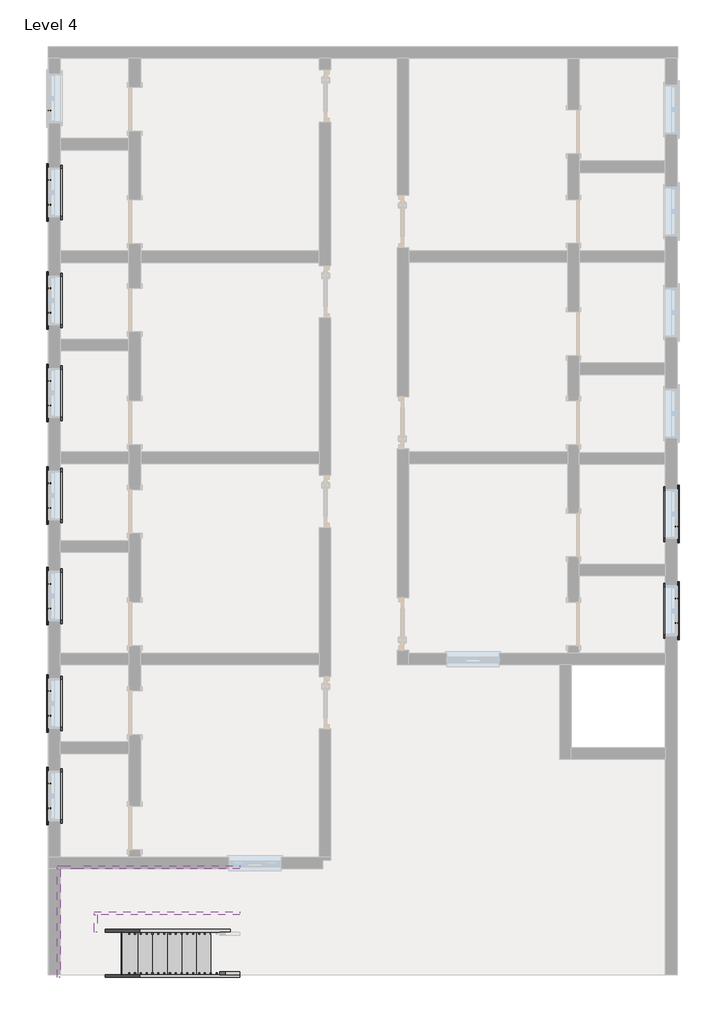
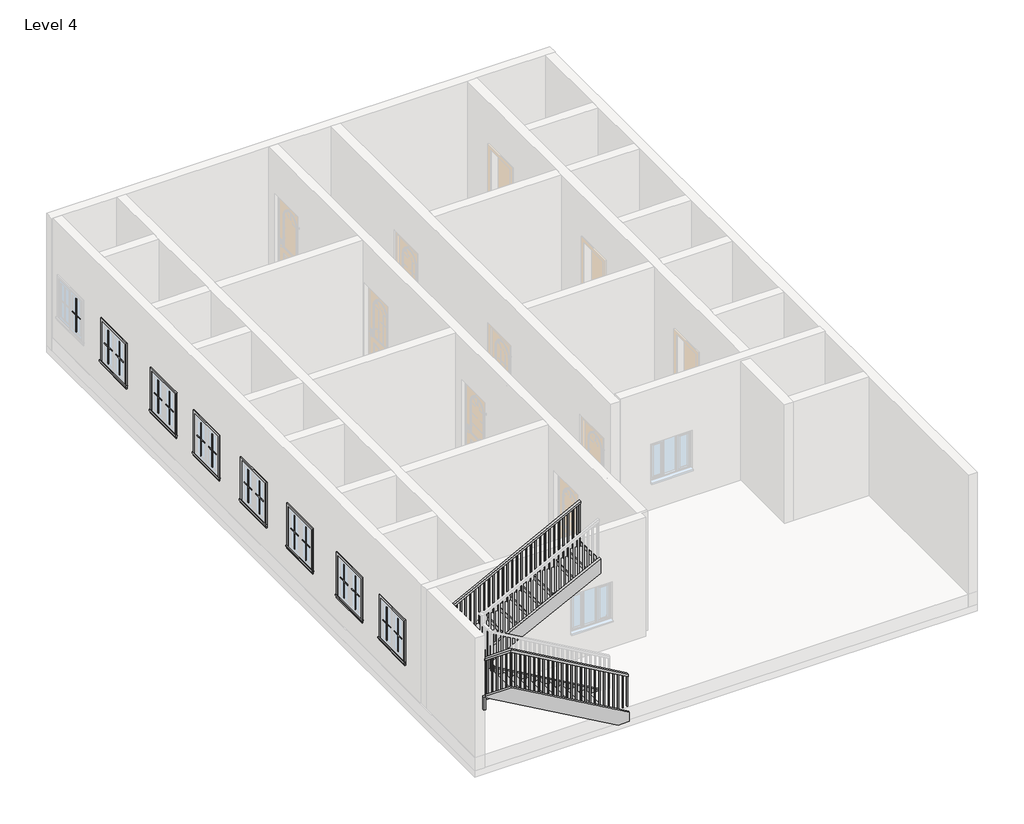
# One storey, part 3 of 4: 36 proxies, 6 members, 1 railing, 1 stair flight.
"""IFC4 building model written with IfcOpenShell, lengths in millimetres."""

from ifc_helpers import new_model, si_unit, frame, origin, place, context, project, spatial, polyline, outline, extrude, faceted_brep, transform, mapped, element, save
from components import muntin_pattern_2x2_muntin_pattern_2x2_b3fe6957, muntin_pattern_2x2_muntin_pattern_2x2_3e0ecaf2, trim_window_exterior_flat_with_sill_41619996, trim_window_interior_flat_picture_frame_51c85655, stair_flight_03342cd4

model = new_model("IFC4")

# Units and contexts
model_context = context("Model", 3, world=origin())
ifc_project = project(units=[si_unit("LENGTHUNIT", "METRE", prefix="MILLI")], contexts=[model_context])

# Site, building, storey
site = spatial("IfcSite", under=ifc_project)
building = spatial("IfcBuilding", under=site)
storey = spatial("IfcBuildingStorey", under=building, Name="Level 4", Elevation=9144.0)

# Proxies
placement = place(None, origin())
muntin_pattern_2x2_muntin_pattern_2x2_shape = muntin_pattern_2x2_muntin_pattern_2x2_b3fe6957(model_context)
element("IfcBuildingElementProxy", 1, Name="Muntin Pattern_2x2 : Muntin Pattern_2x2", ObjectType="Muntin Pattern_2x2 : Muntin Pattern_2x2", at=placement, inside=storey, context=model_context, shape_type="MappedRepresentation", body=[
    mapped(muntin_pattern_2x2_muntin_pattern_2x2_shape, transform((-6438.8858866, 6882.8274728, 10128.25), x_axis=(0.0, 1.0, 0.0), y_axis=(-1.0, 0.0, 0.0), z_axis=(0.0, 0.0, 1.0))),
])
element("IfcBuildingElementProxy", 2, Name="Muntin Pattern_2x2 : Muntin Pattern_2x2", ObjectType="Muntin Pattern_2x2 : Muntin Pattern_2x2", at=placement, inside=storey, context=model_context, shape_type="MappedRepresentation", body=[
    mapped(muntin_pattern_2x2_muntin_pattern_2x2_shape, transform((-6438.8858866, 5244.5274728, 10128.25), x_axis=(0.0, 1.0, 0.0), y_axis=(-1.0, 0.0, 0.0), z_axis=(0.0, 0.0, 1.0))),
])
element("IfcBuildingElementProxy", 3, Name="Muntin Pattern_2x2 : Muntin Pattern_2x2", ObjectType="Muntin Pattern_2x2 : Muntin Pattern_2x2", at=placement, inside=storey, context=model_context, shape_type="MappedRepresentation", body=[
    mapped(muntin_pattern_2x2_muntin_pattern_2x2_shape, transform((-6438.8858866, 3360.4810874, 10128.25), x_axis=(0.0, 1.0, 0.0), y_axis=(-1.0, 0.0, 0.0), z_axis=(0.0, 0.0, 1.0))),
])
element("IfcBuildingElementProxy", 4, Name="Muntin Pattern_2x2 : Muntin Pattern_2x2", ObjectType="Muntin Pattern_2x2 : Muntin Pattern_2x2", at=placement, inside=storey, context=model_context, shape_type="MappedRepresentation", body=[
    mapped(muntin_pattern_2x2_muntin_pattern_2x2_shape, transform((-6438.8858866, 1745.426343, 10128.25), x_axis=(0.0, 1.0, 0.0), y_axis=(-1.0, 0.0, 0.0), z_axis=(0.0, 0.0, 1.0))),
])
element("IfcBuildingElementProxy", 5, Name="Muntin Pattern_2x2 : Muntin Pattern_2x2", ObjectType="Muntin Pattern_2x2 : Muntin Pattern_2x2", at=placement, inside=storey, context=model_context, shape_type="MappedRepresentation", body=[
    mapped(muntin_pattern_2x2_muntin_pattern_2x2_shape, transform((-6438.8858866, -38.6725272, 10128.25), x_axis=(0.0, 1.0, 0.0), y_axis=(-1.0, 0.0, 0.0), z_axis=(0.0, 0.0, 1.0))),
])
element("IfcBuildingElementProxy", 6, Name="Muntin Pattern_2x2 : Muntin Pattern_2x2", ObjectType="Muntin Pattern_2x2 : Muntin Pattern_2x2", at=placement, inside=storey, context=model_context, shape_type="MappedRepresentation", body=[
    mapped(muntin_pattern_2x2_muntin_pattern_2x2_shape, transform((-6438.8858866, -1791.2725272, 10128.25), x_axis=(0.0, 1.0, 0.0), y_axis=(-1.0, 0.0, 0.0), z_axis=(0.0, 0.0, 1.0))),
])
element("IfcBuildingElementProxy", 7, Name="Muntin Pattern_2x2 : Muntin Pattern_2x2", ObjectType="Muntin Pattern_2x2 : Muntin Pattern_2x2", at=placement, inside=storey, context=model_context, shape_type="MappedRepresentation", body=[
    mapped(muntin_pattern_2x2_muntin_pattern_2x2_shape, transform((-6438.8858866, -3658.1725272, 10128.25), x_axis=(0.0, 1.0, 0.0), y_axis=(-1.0, 0.0, 0.0), z_axis=(0.0, 0.0, 1.0))),
])
element("IfcBuildingElementProxy", 8, Name="Muntin Pattern_2x2 : Muntin Pattern_2x2", ObjectType="Muntin Pattern_2x2 : Muntin Pattern_2x2", at=placement, inside=storey, context=model_context, shape_type="MappedRepresentation", body=[
    mapped(muntin_pattern_2x2_muntin_pattern_2x2_shape, transform((-6438.8858866, -5271.0725272, 10128.25), x_axis=(0.0, 1.0, 0.0), y_axis=(-1.0, 0.0, 0.0), z_axis=(0.0, 0.0, 1.0))),
])
element("IfcBuildingElementProxy", 9, Name="Muntin Pattern_2x2 : Muntin Pattern_2x2", ObjectType="Muntin Pattern_2x2 : Muntin Pattern_2x2", at=placement, inside=storey, context=model_context, shape_type="MappedRepresentation", body=[
    mapped(muntin_pattern_2x2_muntin_pattern_2x2_shape, transform((4489.4641134, -1616.6475272, 10128.25), x_axis=(0.0, -1.0, 0.0), y_axis=(1.0, 0.0, 0.0), z_axis=(0.0, 0.0, 1.0))),
])
muntin_pattern_2x2_muntin_pattern_2x2_2_shape = muntin_pattern_2x2_muntin_pattern_2x2_3e0ecaf2(model_context)
element("IfcBuildingElementProxy", 10, Name="Muntin Pattern_2x2 : Muntin Pattern_2x2", ObjectType="Muntin Pattern_2x2 : Muntin Pattern_2x2", at=placement, inside=storey, context=model_context, shape_type="MappedRepresentation", body=[
    mapped(muntin_pattern_2x2_muntin_pattern_2x2_2_shape, transform((-6438.8858866, 5673.1524728, 10128.25), x_axis=(0.0, -1.0, 0.0), y_axis=(1.0, 0.0, 0.0), z_axis=(0.0, 0.0, 1.0))),
])
element("IfcBuildingElementProxy", 11, Name="Muntin Pattern_2x2 : Muntin Pattern_2x2", ObjectType="Muntin Pattern_2x2 : Muntin Pattern_2x2", at=placement, inside=storey, context=model_context, shape_type="MappedRepresentation", body=[
    mapped(muntin_pattern_2x2_muntin_pattern_2x2_2_shape, transform((-6438.8858866, 3789.1060874, 10128.25), x_axis=(0.0, -1.0, 0.0), y_axis=(1.0, 0.0, 0.0), z_axis=(0.0, 0.0, 1.0))),
])
element("IfcBuildingElementProxy", 12, Name="Muntin Pattern_2x2 : Muntin Pattern_2x2", ObjectType="Muntin Pattern_2x2 : Muntin Pattern_2x2", at=placement, inside=storey, context=model_context, shape_type="MappedRepresentation", body=[
    mapped(muntin_pattern_2x2_muntin_pattern_2x2_2_shape, transform((-6438.8858866, 2174.051343, 10128.25), x_axis=(0.0, -1.0, 0.0), y_axis=(1.0, 0.0, 0.0), z_axis=(0.0, 0.0, 1.0))),
])
element("IfcBuildingElementProxy", 13, Name="Muntin Pattern_2x2 : Muntin Pattern_2x2", ObjectType="Muntin Pattern_2x2 : Muntin Pattern_2x2", at=placement, inside=storey, context=model_context, shape_type="MappedRepresentation", body=[
    mapped(muntin_pattern_2x2_muntin_pattern_2x2_2_shape, transform((-6438.8858866, 389.9524728, 10128.25), x_axis=(0.0, -1.0, 0.0), y_axis=(1.0, 0.0, 0.0), z_axis=(0.0, 0.0, 1.0))),
])
element("IfcBuildingElementProxy", 14, Name="Muntin Pattern_2x2 : Muntin Pattern_2x2", ObjectType="Muntin Pattern_2x2 : Muntin Pattern_2x2", at=placement, inside=storey, context=model_context, shape_type="MappedRepresentation", body=[
    mapped(muntin_pattern_2x2_muntin_pattern_2x2_2_shape, transform((-6438.8858866, -1362.6475272, 10128.25), x_axis=(0.0, -1.0, 0.0), y_axis=(1.0, 0.0, 0.0), z_axis=(0.0, 0.0, 1.0))),
])
element("IfcBuildingElementProxy", 15, Name="Muntin Pattern_2x2 : Muntin Pattern_2x2", ObjectType="Muntin Pattern_2x2 : Muntin Pattern_2x2", at=placement, inside=storey, context=model_context, shape_type="MappedRepresentation", body=[
    mapped(muntin_pattern_2x2_muntin_pattern_2x2_2_shape, transform((-6438.8858866, -3229.5475272, 10128.25), x_axis=(0.0, -1.0, 0.0), y_axis=(1.0, 0.0, 0.0), z_axis=(0.0, 0.0, 1.0))),
])
element("IfcBuildingElementProxy", 16, Name="Muntin Pattern_2x2 : Muntin Pattern_2x2", ObjectType="Muntin Pattern_2x2 : Muntin Pattern_2x2", at=placement, inside=storey, context=model_context, shape_type="MappedRepresentation", body=[
    mapped(muntin_pattern_2x2_muntin_pattern_2x2_2_shape, transform((-6438.8858866, -4842.4475272, 10128.25), x_axis=(0.0, -1.0, 0.0), y_axis=(1.0, 0.0, 0.0), z_axis=(0.0, 0.0, 1.0))),
])
element("IfcBuildingElementProxy", 17, Name="Muntin Pattern_2x2 : Muntin Pattern_2x2", ObjectType="Muntin Pattern_2x2 : Muntin Pattern_2x2", at=placement, inside=storey, context=model_context, shape_type="MappedRepresentation", body=[
    mapped(muntin_pattern_2x2_muntin_pattern_2x2_2_shape, transform((4489.4641134, -2045.2725272, 10128.25), x_axis=(0.0, 1.0, 0.0), y_axis=(-1.0, 0.0, 0.0), z_axis=(0.0, 0.0, 1.0))),
])
element("IfcBuildingElementProxy", 18, Name="Muntin Pattern_2x2 : Muntin Pattern_2x2", ObjectType="Muntin Pattern_2x2 : Muntin Pattern_2x2", at=placement, inside=storey, context=model_context, shape_type="MappedRepresentation", body=[
    mapped(muntin_pattern_2x2_muntin_pattern_2x2_2_shape, transform((4489.4641134, -362.5225272, 10128.25), x_axis=(0.0, 1.0, 0.0), y_axis=(-1.0, 0.0, 0.0), z_axis=(0.0, 0.0, 1.0))),
])
trim_window_exterior_flat_with_sill_shape = trim_window_exterior_flat_with_sill_41619996(model_context)
element("IfcBuildingElementProxy", 19, Name="Trim-Window-Exterior-Flat : with Sill", ObjectType="Trim-Window-Exterior-Flat : with Sill", at=placement, inside=storey, context=model_context, shape_type="MappedRepresentation", body=[
    mapped(trim_window_exterior_flat_with_sill_shape, transform((-6448.4108866, 5458.8399728, 10972.8), x_axis=(0.0, -1.0, 0.0), y_axis=(0.0, 0.0, 1.0), z_axis=(-1.0, 0.0, 0.0))),
])
element("IfcBuildingElementProxy", 20, Name="Trim-Window-Exterior-Flat : with Sill", ObjectType="Trim-Window-Exterior-Flat : with Sill", at=placement, inside=storey, context=model_context, shape_type="MappedRepresentation", body=[
    mapped(trim_window_exterior_flat_with_sill_shape, transform((-6448.4108866, 3574.7935874, 10972.8), x_axis=(0.0, -1.0, 0.0), y_axis=(0.0, 0.0, 1.0), z_axis=(-1.0, 0.0, 0.0))),
])
element("IfcBuildingElementProxy", 21, Name="Trim-Window-Exterior-Flat : with Sill", ObjectType="Trim-Window-Exterior-Flat : with Sill", at=placement, inside=storey, context=model_context, shape_type="MappedRepresentation", body=[
    mapped(trim_window_exterior_flat_with_sill_shape, transform((-6448.4108866, 1959.738843, 10972.8), x_axis=(0.0, -1.0, 0.0), y_axis=(0.0, 0.0, 1.0), z_axis=(-1.0, 0.0, 0.0))),
])
element("IfcBuildingElementProxy", 22, Name="Trim-Window-Exterior-Flat : with Sill", ObjectType="Trim-Window-Exterior-Flat : with Sill", at=placement, inside=storey, context=model_context, shape_type="MappedRepresentation", body=[
    mapped(trim_window_exterior_flat_with_sill_shape, transform((-6448.4108866, 175.6399728, 10972.8), x_axis=(0.0, -1.0, 0.0), y_axis=(0.0, 0.0, 1.0), z_axis=(-1.0, 0.0, 0.0))),
])
element("IfcBuildingElementProxy", 23, Name="Trim-Window-Exterior-Flat : with Sill", ObjectType="Trim-Window-Exterior-Flat : with Sill", at=placement, inside=storey, context=model_context, shape_type="MappedRepresentation", body=[
    mapped(trim_window_exterior_flat_with_sill_shape, transform((-6448.4108866, -1576.9600272, 10972.8), x_axis=(0.0, -1.0, 0.0), y_axis=(0.0, 0.0, 1.0), z_axis=(-1.0, 0.0, 0.0))),
])
element("IfcBuildingElementProxy", 24, Name="Trim-Window-Exterior-Flat : with Sill", ObjectType="Trim-Window-Exterior-Flat : with Sill", at=placement, inside=storey, context=model_context, shape_type="MappedRepresentation", body=[
    mapped(trim_window_exterior_flat_with_sill_shape, transform((-6448.4108866, -3443.8600272, 10972.8), x_axis=(0.0, -1.0, 0.0), y_axis=(0.0, 0.0, 1.0), z_axis=(-1.0, 0.0, 0.0))),
])
element("IfcBuildingElementProxy", 25, Name="Trim-Window-Exterior-Flat : with Sill", ObjectType="Trim-Window-Exterior-Flat : with Sill", at=placement, inside=storey, context=model_context, shape_type="MappedRepresentation", body=[
    mapped(trim_window_exterior_flat_with_sill_shape, transform((-6448.4108866, -5056.7600272, 10972.8), x_axis=(0.0, -1.0, 0.0), y_axis=(0.0, 0.0, 1.0), z_axis=(-1.0, 0.0, 0.0))),
])
element("IfcBuildingElementProxy", 26, Name="Trim-Window-Exterior-Flat : with Sill", ObjectType="Trim-Window-Exterior-Flat : with Sill", at=placement, inside=storey, context=model_context, shape_type="MappedRepresentation", body=[
    mapped(trim_window_exterior_flat_with_sill_shape, transform((4498.9891134, -1830.9600272, 10972.8), x_axis=(0.0, 1.0, 0.0), y_axis=(0.0, 0.0, 1.0), z_axis=(1.0, 0.0, 0.0))),
])
element("IfcBuildingElementProxy", 27, Name="Trim-Window-Exterior-Flat : with Sill", ObjectType="Trim-Window-Exterior-Flat : with Sill", at=placement, inside=storey, context=model_context, shape_type="MappedRepresentation", body=[
    mapped(trim_window_exterior_flat_with_sill_shape, transform((4498.9891134, -148.2100272, 10972.8), x_axis=(0.0, 1.0, 0.0), y_axis=(0.0, 0.0, 1.0), z_axis=(1.0, 0.0, 0.0))),
])
trim_window_interior_flat_picture_frame_shape = trim_window_interior_flat_picture_frame_51c85655(model_context)
element("IfcBuildingElementProxy", 28, Name="Trim-Window-Interior-Flat : Picture Frame", ObjectType="Trim-Window-Interior-Flat : Picture Frame", at=placement, inside=storey, context=model_context, shape_type="MappedRepresentation", body=[
    mapped(trim_window_interior_flat_picture_frame_shape, transform((-6245.2108866, 5458.8399728, 10972.8), x_axis=(0.0, 1.0, 0.0), y_axis=(0.0, 0.0, 1.0), z_axis=(1.0, 0.0, 0.0))),
])
element("IfcBuildingElementProxy", 29, Name="Trim-Window-Interior-Flat : Picture Frame", ObjectType="Trim-Window-Interior-Flat : Picture Frame", at=placement, inside=storey, context=model_context, shape_type="MappedRepresentation", body=[
    mapped(trim_window_interior_flat_picture_frame_shape, transform((-6245.2108866, 3574.7935874, 10972.8), x_axis=(0.0, 1.0, 0.0), y_axis=(0.0, 0.0, 1.0), z_axis=(1.0, 0.0, 0.0))),
])
element("IfcBuildingElementProxy", 30, Name="Trim-Window-Interior-Flat : Picture Frame", ObjectType="Trim-Window-Interior-Flat : Picture Frame", at=placement, inside=storey, context=model_context, shape_type="MappedRepresentation", body=[
    mapped(trim_window_interior_flat_picture_frame_shape, transform((-6245.2108866, 1959.738843, 10972.8), x_axis=(0.0, 1.0, 0.0), y_axis=(0.0, 0.0, 1.0), z_axis=(1.0, 0.0, 0.0))),
])
element("IfcBuildingElementProxy", 31, Name="Trim-Window-Interior-Flat : Picture Frame", ObjectType="Trim-Window-Interior-Flat : Picture Frame", at=placement, inside=storey, context=model_context, shape_type="MappedRepresentation", body=[
    mapped(trim_window_interior_flat_picture_frame_shape, transform((-6245.2108866, 175.6399728, 10972.8), x_axis=(0.0, 1.0, 0.0), y_axis=(0.0, 0.0, 1.0), z_axis=(1.0, 0.0, 0.0))),
])
element("IfcBuildingElementProxy", 32, Name="Trim-Window-Interior-Flat : Picture Frame", ObjectType="Trim-Window-Interior-Flat : Picture Frame", at=placement, inside=storey, context=model_context, shape_type="MappedRepresentation", body=[
    mapped(trim_window_interior_flat_picture_frame_shape, transform((-6245.2108866, -1576.9600272, 10972.8), x_axis=(0.0, 1.0, 0.0), y_axis=(0.0, 0.0, 1.0), z_axis=(1.0, 0.0, 0.0))),
])
element("IfcBuildingElementProxy", 33, Name="Trim-Window-Interior-Flat : Picture Frame", ObjectType="Trim-Window-Interior-Flat : Picture Frame", at=placement, inside=storey, context=model_context, shape_type="MappedRepresentation", body=[
    mapped(trim_window_interior_flat_picture_frame_shape, transform((-6245.2108866, -3443.8600272, 10972.8), x_axis=(0.0, 1.0, 0.0), y_axis=(0.0, 0.0, 1.0), z_axis=(1.0, 0.0, 0.0))),
])
element("IfcBuildingElementProxy", 34, Name="Trim-Window-Interior-Flat : Picture Frame", ObjectType="Trim-Window-Interior-Flat : Picture Frame", at=placement, inside=storey, context=model_context, shape_type="MappedRepresentation", body=[
    mapped(trim_window_interior_flat_picture_frame_shape, transform((-6245.2108866, -5056.7600272, 10972.8), x_axis=(0.0, 1.0, 0.0), y_axis=(0.0, 0.0, 1.0), z_axis=(1.0, 0.0, 0.0))),
])
element("IfcBuildingElementProxy", 35, Name="Trim-Window-Interior-Flat : Picture Frame", ObjectType="Trim-Window-Interior-Flat : Picture Frame", at=placement, inside=storey, context=model_context, shape_type="MappedRepresentation", body=[
    mapped(trim_window_interior_flat_picture_frame_shape, transform((4295.7891134, -1830.9600272, 10972.8), x_axis=(0.0, -1.0, 0.0), y_axis=(0.0, 0.0, 1.0), z_axis=(-1.0, 0.0, 0.0))),
])
element("IfcBuildingElementProxy", 36, Name="Trim-Window-Interior-Flat : Picture Frame", ObjectType="Trim-Window-Interior-Flat : Picture Frame", at=placement, inside=storey, context=model_context, shape_type="MappedRepresentation", body=[
    mapped(trim_window_interior_flat_picture_frame_shape, transform((4295.7891134, -148.2100272, 10972.8), x_axis=(0.0, -1.0, 0.0), y_axis=(0.0, 0.0, 1.0), z_axis=(-1.0, 0.0, 0.0))),
])

# Members
element("IfcMember", 37, ObjectType="Stringer - 2\" Width", at=placement, inside=storey, context=model_context, shape_type="SweptSolid", body=[
    extrude(outline(polyline([(9144.0, -3117.2664982), (9352.974685, -3117.2664982), (10816.7714286, -5678.9107995), (10816.7714286, -6245.2108866), (10789.3177409, -6245.2108866), (9144.0, -3365.9048399), (9144.0, -3117.2664982)])), frame((0.0, -8219.0600272, 0.0), z_axis=(0.0, 1.0, 0.0), x_axis=(0.0, 0.0, 1.0)), (0.0, 0.0, 1.0), 50.8),
])
element("IfcMember", 38, ObjectType="Stringer - 2\" Width", at=placement, inside=storey, context=model_context, shape_type="SweptSolid", body=[
    extrude(outline(polyline([(-6245.2108866, -8219.0600272), (-6296.0108866, -8219.0600272), (-6296.0108866, -6326.7600272), (-6245.2108866, -6326.7600272), (-6245.2108866, -8219.0600272)])), frame((0.0, 0.0, 10511.9714286), z_axis=(0.0, 0.0, 1.0), x_axis=(1.0, 0.0, 0.0)), (0.0, 0.0, 1.0), 304.8),
])
element("IfcMember", 39, ObjectType="Stringer - 2\" Width", at=placement, inside=storey, context=model_context, shape_type="SweptSolid", body=[
    extrude(outline(polyline([(10619.8463219, -6296.0108866), (10511.9714286, -6296.0108866), (10511.9714286, -5835.3420022), (11892.5812084, -3117.2664982), (12234.4466461, -3117.2664982), (10619.8463219, -6296.0108866)])), frame((0.0, -6326.7600272, 0.0), z_axis=(0.0, 1.0, 0.0), x_axis=(0.0, 0.0, 1.0)), (0.0, 0.0, 1.0), 50.8),
])
element("IfcMember", 40, ObjectType="Stringer - 2\" Width", at=placement, inside=storey, context=model_context, shape_type="SweptSolid", body=[
    extrude(outline(polyline([(9144.0, -3117.2664982), (9352.974685, -3117.2664982), (10775.374685, -5606.4664982), (10424.3209476, -5606.4664982), (9144.0, -3365.9048399), (9144.0, -3117.2664982)])), frame((0.0, -7431.6600272, 0.0), z_axis=(0.0, 1.0, 0.0), x_axis=(0.0, 0.0, 1.0)), (0.0, 0.0, 1.0), 50.8),
])
element("IfcMember", 41, ObjectType="Stringer - 2\" Width", at=placement, inside=storey, context=model_context, shape_type="SweptSolid", body=[
    extrude(outline(polyline([(-5606.4664982, -7431.6600272), (-5657.2664982, -7431.6600272), (-5657.2664982, -7126.8600272), (-5606.4664982, -7126.8600272), (-5606.4664982, -7431.6600272)])), frame((0.0, 0.0, 10511.9714286), z_axis=(0.0, 0.0, 1.0), x_axis=(1.0, 0.0, 0.0)), (0.0, 0.0, 1.0), 304.8),
])
element("IfcMember", 42, ObjectType="Stringer - 2\" Width", at=placement, inside=storey, context=model_context, shape_type="SweptSolid", body=[
    extrude(outline(polyline([(10944.287916, -5657.2664982), (10602.4224783, -5657.2664982), (11892.5812084, -3117.2664982), (12234.4466461, -3117.2664982), (10944.287916, -5657.2664982)])), frame((0.0, -7126.8600272, 0.0), z_axis=(0.0, 1.0, 0.0), x_axis=(0.0, 0.0, 1.0)), (0.0, 0.0, 1.0), 50.8),
])

# Railing
element("IfcRailing", 43, ObjectType="Handrail - Rectangular", at=placement, inside=storey, context=model_context, shape_type="SolidModel", body=[
    faceted_brep([(-3117.2664982, -8168.2600272, 10203.5428571), (-3117.2664982, -8168.2600272, 10145.0339009), (-3117.2664982, -8117.4600272, 10145.0339009), (-3117.2664982, -8117.4600272, 10203.5428571), (-5657.2664982, -8168.2600272, 11654.9714286), (-5670.7571716, -8168.2600272, 11604.1714286), (-5670.7571716, -8117.4600272, 11604.1714286), (-5657.2664982, -8117.4600272, 11654.9714286), (-6245.2108866, -8168.2600272, 11654.9714286), (-6245.2108866, -8168.2600272, 11604.1714286), (-6194.4108866, -8117.4600272, 11604.1714286), (-6194.4108866, -8117.4600272, 11654.9714286), (-6245.2108866, -6326.7600272, 11654.9714286), (-6245.2108866, -6326.7600272, 11604.1714286), (-6194.4108866, -6377.5600272, 11604.1714286), (-6194.4108866, -6377.5600272, 11654.9714286), (-5939.4887204, -6326.7600272, 11654.9714286), (-5927.1913462, -6326.7600272, 11604.1714286), (-5927.1913462, -6377.5600272, 11604.1714286), (-5939.4887204, -6377.5600272, 11654.9714286), (-3117.2664982, -6326.7600272, 13106.4), (-3117.2664982, -6377.5600272, 13106.4), (-3117.2664982, -6377.5600272, 13049.2756361), (-3117.2664982, -6326.7600272, 13049.2756361)], [[[0, 1, 2, 3]], [[1, 0, 4, 5]], [[2, 1, 5, 6]], [[3, 2, 6, 7]], [[0, 3, 7, 4]], [[5, 4, 8, 9]], [[6, 5, 9, 10]], [[7, 6, 10, 11]], [[4, 7, 11, 8]], [[9, 8, 12, 13]], [[10, 9, 13, 14]], [[11, 10, 14, 15]], [[8, 11, 15, 12]], [[13, 12, 16, 17]], [[14, 13, 17, 18]], [[15, 14, 18, 19]], [[12, 15, 19, 16]], [[20, 21, 22, 23]], [[17, 16, 20, 23]], [[18, 17, 23, 22]], [[19, 18, 22, 21]], [[16, 19, 21, 20]]]),
    extrude(outline(polyline([(13016.325665, -3181.3358866), (12046.8571429, -3181.3358866), (12046.8571429, -3162.2858866), (13026.1228078, -3162.2858866), (13016.325665, -3181.3358866)])), frame((0.0, -6361.6850272, 0.0), z_axis=(0.0, 1.0, 0.0), x_axis=(0.0, 0.0, 1.0)), (0.0, 0.0, 1.0), 19.05),
    extrude(outline(polyline([(12964.0742364, -3282.9358866), (12046.8571429, -3282.9358866), (12046.8571429, -3263.8858866), (12973.8713793, -3263.8858866), (12964.0742364, -3282.9358866)])), frame((0.0, -6361.6850272, 0.0), z_axis=(0.0, 1.0, 0.0), x_axis=(0.0, 0.0, 1.0)), (0.0, 0.0, 1.0), 19.05),
    extrude(outline(polyline([(12911.8228078, -3384.5358866), (11901.7142857, -3384.5358866), (11901.7142857, -3365.4858866), (12921.6199507, -3365.4858866), (12911.8228078, -3384.5358866)])), frame((0.0, -6361.6850272, 0.0), z_axis=(0.0, 1.0, 0.0), x_axis=(0.0, 0.0, 1.0)), (0.0, 0.0, 1.0), 19.05),
    extrude(outline(polyline([(12859.5713793, -3486.1358866), (11901.7142857, -3486.1358866), (11901.7142857, -3467.0858866), (12869.3685221, -3467.0858866), (12859.5713793, -3486.1358866)])), frame((0.0, -6361.6850272, 0.0), z_axis=(0.0, 1.0, 0.0), x_axis=(0.0, 0.0, 1.0)), (0.0, 0.0, 1.0), 19.05),
    extrude(outline(polyline([(12807.3199507, -3587.7358866), (11901.7142857, -3587.7358866), (11901.7142857, -3568.6858866), (12817.1170935, -3568.6858866), (12807.3199507, -3587.7358866)])), frame((0.0, -6361.6850272, 0.0), z_axis=(0.0, 1.0, 0.0), x_axis=(0.0, 0.0, 1.0)), (0.0, 0.0, 1.0), 19.05),
    extrude(outline(polyline([(12755.0685221, -3689.3358866), (11756.5714286, -3689.3358866), (11756.5714286, -3670.2858866), (12764.865665, -3670.2858866), (12755.0685221, -3689.3358866)])), frame((0.0, -6361.6850272, 0.0), z_axis=(0.0, 1.0, 0.0), x_axis=(0.0, 0.0, 1.0)), (0.0, 0.0, 1.0), 19.05),
    extrude(outline(polyline([(12702.8170935, -3790.9358866), (11756.5714286, -3790.9358866), (11756.5714286, -3771.8858866), (12712.6142364, -3771.8858866), (12702.8170935, -3790.9358866)])), frame((0.0, -6361.6850272, 0.0), z_axis=(0.0, 1.0, 0.0), x_axis=(0.0, 0.0, 1.0)), (0.0, 0.0, 1.0), 19.05),
    extrude(outline(polyline([(12650.565665, -3892.5358866), (11756.5714286, -3892.5358866), (11756.5714286, -3873.4858866), (12660.3628078, -3873.4858866), (12650.565665, -3892.5358866)])), frame((0.0, -6361.6850272, 0.0), z_axis=(0.0, 1.0, 0.0), x_axis=(0.0, 0.0, 1.0)), (0.0, 0.0, 1.0), 19.05),
    extrude(outline(polyline([(12598.3142364, -3994.1358866), (11756.5714286, -3994.1358866), (11756.5714286, -3975.0858866), (12608.1113793, -3975.0858866), (12598.3142364, -3994.1358866)])), frame((0.0, -6361.6850272, 0.0), z_axis=(0.0, 1.0, 0.0), x_axis=(0.0, 0.0, 1.0)), (0.0, 0.0, 1.0), 19.05),
    extrude(outline(polyline([(12546.0628078, -4095.7358866), (11756.5714286, -4095.7358866), (11756.5714286, -4076.6858866), (12555.8599507, -4076.6858866), (12546.0628078, -4095.7358866)])), frame((0.0, -6361.6850272, 0.0), z_axis=(0.0, 1.0, 0.0), x_axis=(0.0, 0.0, 1.0)), (0.0, 0.0, 1.0), 19.05),
    extrude(outline(polyline([(12493.8113793, -4197.3358866), (11611.4285714, -4197.3358866), (11611.4285714, -4178.2858866), (12503.6085221, -4178.2858866), (12493.8113793, -4197.3358866)])), frame((0.0, -6361.6850272, 0.0), z_axis=(0.0, 1.0, 0.0), x_axis=(0.0, 0.0, 1.0)), (0.0, 0.0, 1.0), 19.05),
    extrude(outline(polyline([(12441.5599507, -4298.9358866), (11611.4285714, -4298.9358866), (11611.4285714, -4279.8858866), (12451.3570935, -4279.8858866), (12441.5599507, -4298.9358866)])), frame((0.0, -6361.6850272, 0.0), z_axis=(0.0, 1.0, 0.0), x_axis=(0.0, 0.0, 1.0)), (0.0, 0.0, 1.0), 19.05),
    extrude(outline(polyline([(12389.3085221, -4400.5358866), (11466.2857143, -4400.5358866), (11466.2857143, -4381.4858866), (12399.105665, -4381.4858866), (12389.3085221, -4400.5358866)])), frame((0.0, -6361.6850272, 0.0), z_axis=(0.0, 1.0, 0.0), x_axis=(0.0, 0.0, 1.0)), (0.0, 0.0, 1.0), 19.05),
    extrude(outline(polyline([(12337.0570935, -4502.1358866), (11466.2857143, -4502.1358866), (11466.2857143, -4483.0858866), (12346.8542364, -4483.0858866), (12337.0570935, -4502.1358866)])), frame((0.0, -6361.6850272, 0.0), z_axis=(0.0, 1.0, 0.0), x_axis=(0.0, 0.0, 1.0)), (0.0, 0.0, 1.0), 19.05),
    extrude(outline(polyline([(12284.805665, -4603.7358866), (11466.2857143, -4603.7358866), (11466.2857143, -4584.6858866), (12294.6028078, -4584.6858866), (12284.805665, -4603.7358866)])), frame((0.0, -6361.6850272, 0.0), z_axis=(0.0, 1.0, 0.0), x_axis=(0.0, 0.0, 1.0)), (0.0, 0.0, 1.0), 19.05),
    extrude(outline(polyline([(12232.5542364, -4705.3358866), (11321.1428571, -4705.3358866), (11321.1428571, -4686.2858866), (12242.3513793, -4686.2858866), (12232.5542364, -4705.3358866)])), frame((0.0, -6361.6850272, 0.0), z_axis=(0.0, 1.0, 0.0), x_axis=(0.0, 0.0, 1.0)), (0.0, 0.0, 1.0), 19.05),
    extrude(outline(polyline([(12180.3028078, -4806.9358866), (11321.1428571, -4806.9358866), (11321.1428571, -4787.8858866), (12190.0999507, -4787.8858866), (12180.3028078, -4806.9358866)])), frame((0.0, -6361.6850272, 0.0), z_axis=(0.0, 1.0, 0.0), x_axis=(0.0, 0.0, 1.0)), (0.0, 0.0, 1.0), 19.05),
    extrude(outline(polyline([(12128.0513793, -4908.5358866), (11176.0, -4908.5358866), (11176.0, -4889.4858866), (12137.8485221, -4889.4858866), (12128.0513793, -4908.5358866)])), frame((0.0, -6361.6850272, 0.0), z_axis=(0.0, 1.0, 0.0), x_axis=(0.0, 0.0, 1.0)), (0.0, 0.0, 1.0), 19.05),
    extrude(outline(polyline([(12075.7999507, -5010.1358866), (11176.0, -5010.1358866), (11176.0, -4991.0858866), (12085.5970935, -4991.0858866), (12075.7999507, -5010.1358866)])), frame((0.0, -6361.6850272, 0.0), z_axis=(0.0, 1.0, 0.0), x_axis=(0.0, 0.0, 1.0)), (0.0, 0.0, 1.0), 19.05),
    extrude(outline(polyline([(12023.5485221, -5111.7358866), (11176.0, -5111.7358866), (11176.0, -5092.6858866), (12033.345665, -5092.6858866), (12023.5485221, -5111.7358866)])), frame((0.0, -6361.6850272, 0.0), z_axis=(0.0, 1.0, 0.0), x_axis=(0.0, 0.0, 1.0)), (0.0, 0.0, 1.0), 19.05),
    extrude(outline(polyline([(11971.2970935, -5213.3358866), (11030.8571429, -5213.3358866), (11030.8571429, -5194.2858866), (11981.0942364, -5194.2858866), (11971.2970935, -5213.3358866)])), frame((0.0, -6361.6850272, 0.0), z_axis=(0.0, 1.0, 0.0), x_axis=(0.0, 0.0, 1.0)), (0.0, 0.0, 1.0), 19.05),
    extrude(outline(polyline([(11919.045665, -5314.9358866), (11030.8571429, -5314.9358866), (11030.8571429, -5295.8858866), (11928.8428078, -5295.8858866), (11919.045665, -5314.9358866)])), frame((0.0, -6361.6850272, 0.0), z_axis=(0.0, 1.0, 0.0), x_axis=(0.0, 0.0, 1.0)), (0.0, 0.0, 1.0), 19.05),
    extrude(outline(polyline([(11866.7942364, -5416.5358866), (10885.7142857, -5416.5358866), (10885.7142857, -5397.4858866), (11876.5913793, -5397.4858866), (11866.7942364, -5416.5358866)])), frame((0.0, -6361.6850272, 0.0), z_axis=(0.0, 1.0, 0.0), x_axis=(0.0, 0.0, 1.0)), (0.0, 0.0, 1.0), 19.05),
    extrude(outline(polyline([(11814.5428078, -5518.1358866), (10885.7142857, -5518.1358866), (10885.7142857, -5499.0858866), (11824.3399507, -5499.0858866), (11814.5428078, -5518.1358866)])), frame((0.0, -6361.6850272, 0.0), z_axis=(0.0, 1.0, 0.0), x_axis=(0.0, 0.0, 1.0)), (0.0, 0.0, 1.0), 19.05),
    extrude(outline(polyline([(11762.2913793, -5619.7358866), (10885.7142857, -5619.7358866), (10885.7142857, -5600.6858866), (11772.0885221, -5600.6858866), (11762.2913793, -5619.7358866)])), frame((0.0, -6361.6850272, 0.0), z_axis=(0.0, 1.0, 0.0), x_axis=(0.0, 0.0, 1.0)), (0.0, 0.0, 1.0), 19.05),
    extrude(outline(polyline([(11710.0399507, -5721.3358866), (10740.5714286, -5721.3358866), (10740.5714286, -5702.2858866), (11719.8370935, -5702.2858866), (11710.0399507, -5721.3358866)])), frame((0.0, -6361.6850272, 0.0), z_axis=(0.0, 1.0, 0.0), x_axis=(0.0, 0.0, 1.0)), (0.0, 0.0, 1.0), 19.05),
    extrude(outline(polyline([(11657.7885221, -5822.9358866), (10740.5714286, -5822.9358866), (10740.5714286, -5803.8858866), (11667.585665, -5803.8858866), (11657.7885221, -5822.9358866)])), frame((0.0, -6361.6850272, 0.0), z_axis=(0.0, 1.0, 0.0), x_axis=(0.0, 0.0, 1.0)), (0.0, 0.0, 1.0), 19.05),
    extrude(outline(polyline([(11605.5370935, -5924.5358866), (10740.5714286, -5924.5358866), (10740.5714286, -5905.4858866), (11615.3342364, -5905.4858866), (11605.5370935, -5924.5358866)])), frame((0.0, -6361.6850272, 0.0), z_axis=(0.0, 1.0, 0.0), x_axis=(0.0, 0.0, 1.0)), (0.0, 0.0, 1.0), 19.05),
    extrude(outline(polyline([(-6026.1358866, -6342.6350272), (-6007.0858866, -6342.6350272), (-6007.0858866, -6361.6850272), (-6026.1358866, -6361.6850272), (-6026.1358866, -6342.6350272)])), frame((0.0, 0.0, 10740.5714286), z_axis=(0.0, 0.0, 1.0), x_axis=(1.0, 0.0, 0.0)), (0.0, 0.0, 1.0), 863.6),
    extrude(outline(polyline([(-6127.7358866, -6342.6350272), (-6108.6858866, -6342.6350272), (-6108.6858866, -6361.6850272), (-6127.7358866, -6361.6850272), (-6127.7358866, -6342.6350272)])), frame((0.0, 0.0, 10740.5714286), z_axis=(0.0, 0.0, 1.0), x_axis=(1.0, 0.0, 0.0)), (0.0, 0.0, 1.0), 863.6),
    extrude(outline(polyline([(-6229.3358866, -6425.1850272), (-6229.3358866, -6406.1350272), (-6210.2858866, -6406.1350272), (-6210.2858866, -6425.1850272), (-6229.3358866, -6425.1850272)])), frame((0.0, 0.0, 10740.5714286), z_axis=(0.0, 0.0, 1.0), x_axis=(1.0, 0.0, 0.0)), (0.0, 0.0, 1.0), 863.6),
    extrude(outline(polyline([(-6229.3358866, -6526.7850272), (-6229.3358866, -6507.7350272), (-6210.2858866, -6507.7350272), (-6210.2858866, -6526.7850272), (-6229.3358866, -6526.7850272)])), frame((0.0, 0.0, 10740.5714286), z_axis=(0.0, 0.0, 1.0), x_axis=(1.0, 0.0, 0.0)), (0.0, 0.0, 1.0), 863.6),
    extrude(outline(polyline([(-6229.3358866, -6628.3850272), (-6229.3358866, -6609.3350272), (-6210.2858866, -6609.3350272), (-6210.2858866, -6628.3850272), (-6229.3358866, -6628.3850272)])), frame((0.0, 0.0, 10740.5714286), z_axis=(0.0, 0.0, 1.0), x_axis=(1.0, 0.0, 0.0)), (0.0, 0.0, 1.0), 863.6),
    extrude(outline(polyline([(-6229.3358866, -6729.9850272), (-6229.3358866, -6710.9350272), (-6210.2858866, -6710.9350272), (-6210.2858866, -6729.9850272), (-6229.3358866, -6729.9850272)])), frame((0.0, 0.0, 10740.5714286), z_axis=(0.0, 0.0, 1.0), x_axis=(1.0, 0.0, 0.0)), (0.0, 0.0, 1.0), 863.6),
    extrude(outline(polyline([(-6229.3358866, -6831.5850272), (-6229.3358866, -6812.5350272), (-6210.2858866, -6812.5350272), (-6210.2858866, -6831.5850272), (-6229.3358866, -6831.5850272)])), frame((0.0, 0.0, 10740.5714286), z_axis=(0.0, 0.0, 1.0), x_axis=(1.0, 0.0, 0.0)), (0.0, 0.0, 1.0), 863.6),
    extrude(outline(polyline([(-6229.3358866, -6933.1850272), (-6229.3358866, -6914.1350272), (-6210.2858866, -6914.1350272), (-6210.2858866, -6933.1850272), (-6229.3358866, -6933.1850272)])), frame((0.0, 0.0, 10740.5714286), z_axis=(0.0, 0.0, 1.0), x_axis=(1.0, 0.0, 0.0)), (0.0, 0.0, 1.0), 863.6),
    extrude(outline(polyline([(-6229.3358866, -7034.7850272), (-6229.3358866, -7015.7350272), (-6210.2858866, -7015.7350272), (-6210.2858866, -7034.7850272), (-6229.3358866, -7034.7850272)])), frame((0.0, 0.0, 10740.5714286), z_axis=(0.0, 0.0, 1.0), x_axis=(1.0, 0.0, 0.0)), (0.0, 0.0, 1.0), 863.6),
    extrude(outline(polyline([(-6229.3358866, -7136.3850272), (-6229.3358866, -7117.3350272), (-6210.2858866, -7117.3350272), (-6210.2858866, -7136.3850272), (-6229.3358866, -7136.3850272)])), frame((0.0, 0.0, 10740.5714286), z_axis=(0.0, 0.0, 1.0), x_axis=(1.0, 0.0, 0.0)), (0.0, 0.0, 1.0), 863.6),
    extrude(outline(polyline([(-6229.3358866, -7237.9850272), (-6229.3358866, -7218.9350272), (-6210.2858866, -7218.9350272), (-6210.2858866, -7237.9850272), (-6229.3358866, -7237.9850272)])), frame((0.0, 0.0, 10740.5714286), z_axis=(0.0, 0.0, 1.0), x_axis=(1.0, 0.0, 0.0)), (0.0, 0.0, 1.0), 863.6),
    extrude(outline(polyline([(-6229.3358866, -7339.5850272), (-6229.3358866, -7320.5350272), (-6210.2858866, -7320.5350272), (-6210.2858866, -7339.5850272), (-6229.3358866, -7339.5850272)])), frame((0.0, 0.0, 10740.5714286), z_axis=(0.0, 0.0, 1.0), x_axis=(1.0, 0.0, 0.0)), (0.0, 0.0, 1.0), 863.6),
    extrude(outline(polyline([(-6229.3358866, -7441.1850272), (-6229.3358866, -7422.1350272), (-6210.2858866, -7422.1350272), (-6210.2858866, -7441.1850272), (-6229.3358866, -7441.1850272)])), frame((0.0, 0.0, 10740.5714286), z_axis=(0.0, 0.0, 1.0), x_axis=(1.0, 0.0, 0.0)), (0.0, 0.0, 1.0), 863.6),
    extrude(outline(polyline([(-6229.3358866, -7542.7850272), (-6229.3358866, -7523.7350272), (-6210.2858866, -7523.7350272), (-6210.2858866, -7542.7850272), (-6229.3358866, -7542.7850272)])), frame((0.0, 0.0, 10740.5714286), z_axis=(0.0, 0.0, 1.0), x_axis=(1.0, 0.0, 0.0)), (0.0, 0.0, 1.0), 863.6),
    extrude(outline(polyline([(-6229.3358866, -7644.3850272), (-6229.3358866, -7625.3350272), (-6210.2858866, -7625.3350272), (-6210.2858866, -7644.3850272), (-6229.3358866, -7644.3850272)])), frame((0.0, 0.0, 10740.5714286), z_axis=(0.0, 0.0, 1.0), x_axis=(1.0, 0.0, 0.0)), (0.0, 0.0, 1.0), 863.6),
    extrude(outline(polyline([(-6229.3358866, -7745.9850272), (-6229.3358866, -7726.9350272), (-6210.2858866, -7726.9350272), (-6210.2858866, -7745.9850272), (-6229.3358866, -7745.9850272)])), frame((0.0, 0.0, 10740.5714286), z_axis=(0.0, 0.0, 1.0), x_axis=(1.0, 0.0, 0.0)), (0.0, 0.0, 1.0), 863.6),
    extrude(outline(polyline([(-6229.3358866, -7847.5850272), (-6229.3358866, -7828.5350272), (-6210.2858866, -7828.5350272), (-6210.2858866, -7847.5850272), (-6229.3358866, -7847.5850272)])), frame((0.0, 0.0, 10740.5714286), z_axis=(0.0, 0.0, 1.0), x_axis=(1.0, 0.0, 0.0)), (0.0, 0.0, 1.0), 863.6),
    extrude(outline(polyline([(-6229.3358866, -7949.1850272), (-6229.3358866, -7930.1350272), (-6210.2858866, -7930.1350272), (-6210.2858866, -7949.1850272), (-6229.3358866, -7949.1850272)])), frame((0.0, 0.0, 10740.5714286), z_axis=(0.0, 0.0, 1.0), x_axis=(1.0, 0.0, 0.0)), (0.0, 0.0, 1.0), 863.6),
    extrude(outline(polyline([(-6229.3358866, -8050.7850272), (-6229.3358866, -8031.7350272), (-6210.2858866, -8031.7350272), (-6210.2858866, -8050.7850272), (-6229.3358866, -8050.7850272)])), frame((0.0, 0.0, 10740.5714286), z_axis=(0.0, 0.0, 1.0), x_axis=(1.0, 0.0, 0.0)), (0.0, 0.0, 1.0), 863.6),
    extrude(outline(polyline([(-6155.7414982, -8152.3850272), (-6174.7914982, -8152.3850272), (-6174.7914982, -8133.3350272), (-6155.7414982, -8133.3350272), (-6155.7414982, -8152.3850272)])), frame((0.0, 0.0, 10740.5714286), z_axis=(0.0, 0.0, 1.0), x_axis=(1.0, 0.0, 0.0)), (0.0, 0.0, 1.0), 863.6),
    extrude(outline(polyline([(-6054.1414982, -8152.3850272), (-6073.1914982, -8152.3850272), (-6073.1914982, -8133.3350272), (-6054.1414982, -8133.3350272), (-6054.1414982, -8152.3850272)])), frame((0.0, 0.0, 10740.5714286), z_axis=(0.0, 0.0, 1.0), x_axis=(1.0, 0.0, 0.0)), (0.0, 0.0, 1.0), 863.6),
    extrude(outline(polyline([(-5952.5414982, -8152.3850272), (-5971.5914982, -8152.3850272), (-5971.5914982, -8133.3350272), (-5952.5414982, -8133.3350272), (-5952.5414982, -8152.3850272)])), frame((0.0, 0.0, 10740.5714286), z_axis=(0.0, 0.0, 1.0), x_axis=(1.0, 0.0, 0.0)), (0.0, 0.0, 1.0), 863.6),
    extrude(outline(polyline([(-5850.9414982, -8152.3850272), (-5869.9914982, -8152.3850272), (-5869.9914982, -8133.3350272), (-5850.9414982, -8133.3350272), (-5850.9414982, -8152.3850272)])), frame((0.0, 0.0, 10740.5714286), z_axis=(0.0, 0.0, 1.0), x_axis=(1.0, 0.0, 0.0)), (0.0, 0.0, 1.0), 863.6),
    extrude(outline(polyline([(-5749.3414982, -8152.3850272), (-5768.3914982, -8152.3850272), (-5768.3914982, -8133.3350272), (-5749.3414982, -8133.3350272), (-5749.3414982, -8152.3850272)])), frame((0.0, 0.0, 10740.5714286), z_axis=(0.0, 0.0, 1.0), x_axis=(1.0, 0.0, 0.0)), (0.0, 0.0, 1.0), 863.6),
    extrude(outline(polyline([(11601.9053295, -5666.7914982), (10740.5714286, -5666.7914982), (10740.5714286, -5647.7414982), (11591.0196152, -5647.7414982), (11601.9053295, -5666.7914982)])), frame((0.0, -8152.3850272, 0.0), z_axis=(0.0, 1.0, 0.0), x_axis=(0.0, 0.0, 1.0)), (0.0, 0.0, 1.0), 19.05),
    extrude(outline(polyline([(11543.8481866, -5565.1914982), (10595.4285714, -5565.1914982), (10595.4285714, -5546.1414982), (11532.9624723, -5546.1414982), (11543.8481866, -5565.1914982)])), frame((0.0, -8152.3850272, 0.0), z_axis=(0.0, 1.0, 0.0), x_axis=(0.0, 0.0, 1.0)), (0.0, 0.0, 1.0), 19.05),
    extrude(outline(polyline([(11485.7910438, -5463.5914982), (10595.4285714, -5463.5914982), (10595.4285714, -5444.5414982), (11474.9053295, -5444.5414982), (11485.7910438, -5463.5914982)])), frame((0.0, -8152.3850272, 0.0), z_axis=(0.0, 1.0, 0.0), x_axis=(0.0, 0.0, 1.0)), (0.0, 0.0, 1.0), 19.05),
    extrude(outline(polyline([(11427.7339009, -5361.9914982), (10450.2857143, -5361.9914982), (10450.2857143, -5342.9414982), (11416.8481866, -5342.9414982), (11427.7339009, -5361.9914982)])), frame((0.0, -8152.3850272, 0.0), z_axis=(0.0, 1.0, 0.0), x_axis=(0.0, 0.0, 1.0)), (0.0, 0.0, 1.0), 19.05),
    extrude(outline(polyline([(11369.6767581, -5260.3914982), (10450.2857143, -5260.3914982), (10450.2857143, -5241.3414982), (11358.7910438, -5241.3414982), (11369.6767581, -5260.3914982)])), frame((0.0, -8152.3850272, 0.0), z_axis=(0.0, 1.0, 0.0), x_axis=(0.0, 0.0, 1.0)), (0.0, 0.0, 1.0), 19.05),
    extrude(outline(polyline([(11311.6196152, -5158.7914982), (10450.2857143, -5158.7914982), (10450.2857143, -5139.7414982), (11300.7339009, -5139.7414982), (11311.6196152, -5158.7914982)])), frame((0.0, -8152.3850272, 0.0), z_axis=(0.0, 1.0, 0.0), x_axis=(0.0, 0.0, 1.0)), (0.0, 0.0, 1.0), 19.05),
    extrude(outline(polyline([(11253.5624723, -5057.1914982), (10305.1428571, -5057.1914982), (10305.1428571, -5038.1414982), (11242.6767581, -5038.1414982), (11253.5624723, -5057.1914982)])), frame((0.0, -8152.3850272, 0.0), z_axis=(0.0, 1.0, 0.0), x_axis=(0.0, 0.0, 1.0)), (0.0, 0.0, 1.0), 19.05),
    extrude(outline(polyline([(11195.5053295, -4955.5914982), (10305.1428571, -4955.5914982), (10305.1428571, -4936.5414982), (11184.6196152, -4936.5414982), (11195.5053295, -4955.5914982)])), frame((0.0, -8152.3850272, 0.0), z_axis=(0.0, 1.0, 0.0), x_axis=(0.0, 0.0, 1.0)), (0.0, 0.0, 1.0), 19.05),
    extrude(outline(polyline([(11137.4481866, -4853.9914982), (10160.0, -4853.9914982), (10160.0, -4834.9414982), (11126.5624723, -4834.9414982), (11137.4481866, -4853.9914982)])), frame((0.0, -8152.3850272, 0.0), z_axis=(0.0, 1.0, 0.0), x_axis=(0.0, 0.0, 1.0)), (0.0, 0.0, 1.0), 19.05),
    extrude(outline(polyline([(11079.3910438, -4752.3914982), (10160.0, -4752.3914982), (10160.0, -4733.3414982), (11068.5053295, -4733.3414982), (11079.3910438, -4752.3914982)])), frame((0.0, -8152.3850272, 0.0), z_axis=(0.0, 1.0, 0.0), x_axis=(0.0, 0.0, 1.0)), (0.0, 0.0, 1.0), 19.05),
    extrude(outline(polyline([(11021.3339009, -4650.7914982), (10160.0, -4650.7914982), (10160.0, -4631.7414982), (11010.4481866, -4631.7414982), (11021.3339009, -4650.7914982)])), frame((0.0, -8152.3850272, 0.0), z_axis=(0.0, 1.0, 0.0), x_axis=(0.0, 0.0, 1.0)), (0.0, 0.0, 1.0), 19.05),
    extrude(outline(polyline([(10963.2767581, -4549.1914982), (10014.8571429, -4549.1914982), (10014.8571429, -4530.1414982), (10952.3910438, -4530.1414982), (10963.2767581, -4549.1914982)])), frame((0.0, -8152.3850272, 0.0), z_axis=(0.0, 1.0, 0.0), x_axis=(0.0, 0.0, 1.0)), (0.0, 0.0, 1.0), 19.05),
    extrude(outline(polyline([(10905.2196152, -4447.5914982), (10014.8571429, -4447.5914982), (10014.8571429, -4428.5414982), (10894.3339009, -4428.5414982), (10905.2196152, -4447.5914982)])), frame((0.0, -8152.3850272, 0.0), z_axis=(0.0, 1.0, 0.0), x_axis=(0.0, 0.0, 1.0)), (0.0, 0.0, 1.0), 19.05),
    extrude(outline(polyline([(10847.1624723, -4345.9914982), (9869.7142857, -4345.9914982), (9869.7142857, -4326.9414982), (10836.2767581, -4326.9414982), (10847.1624723, -4345.9914982)])), frame((0.0, -8152.3850272, 0.0), z_axis=(0.0, 1.0, 0.0), x_axis=(0.0, 0.0, 1.0)), (0.0, 0.0, 1.0), 19.05),
    extrude(outline(polyline([(10789.1053295, -4244.3914982), (9869.7142857, -4244.3914982), (9869.7142857, -4225.3414982), (10778.2196152, -4225.3414982), (10789.1053295, -4244.3914982)])), frame((0.0, -8152.3850272, 0.0), z_axis=(0.0, 1.0, 0.0), x_axis=(0.0, 0.0, 1.0)), (0.0, 0.0, 1.0), 19.05),
    extrude(outline(polyline([(10731.0481866, -4142.7914982), (9869.7142857, -4142.7914982), (9869.7142857, -4123.7414982), (10720.1624723, -4123.7414982), (10731.0481866, -4142.7914982)])), frame((0.0, -8152.3850272, 0.0), z_axis=(0.0, 1.0, 0.0), x_axis=(0.0, 0.0, 1.0)), (0.0, 0.0, 1.0), 19.05),
    extrude(outline(polyline([(10672.9910438, -4041.1914982), (9724.5714286, -4041.1914982), (9724.5714286, -4022.1414982), (10662.1053295, -4022.1414982), (10672.9910438, -4041.1914982)])), frame((0.0, -8152.3850272, 0.0), z_axis=(0.0, 1.0, 0.0), x_axis=(0.0, 0.0, 1.0)), (0.0, 0.0, 1.0), 19.05),
    extrude(outline(polyline([(10614.9339009, -3939.5914982), (9724.5714286, -3939.5914982), (9724.5714286, -3920.5414982), (10604.0481866, -3920.5414982), (10614.9339009, -3939.5914982)])), frame((0.0, -8152.3850272, 0.0), z_axis=(0.0, 1.0, 0.0), x_axis=(0.0, 0.0, 1.0)), (0.0, 0.0, 1.0), 19.05),
    extrude(outline(polyline([(10556.8767581, -3837.9914982), (9579.4285714, -3837.9914982), (9579.4285714, -3818.9414982), (10545.9910438, -3818.9414982), (10556.8767581, -3837.9914982)])), frame((0.0, -8152.3850272, 0.0), z_axis=(0.0, 1.0, 0.0), x_axis=(0.0, 0.0, 1.0)), (0.0, 0.0, 1.0), 19.05),
    extrude(outline(polyline([(10498.8196152, -3736.3914982), (9579.4285714, -3736.3914982), (9579.4285714, -3717.3414982), (10487.9339009, -3717.3414982), (10498.8196152, -3736.3914982)])), frame((0.0, -8152.3850272, 0.0), z_axis=(0.0, 1.0, 0.0), x_axis=(0.0, 0.0, 1.0)), (0.0, 0.0, 1.0), 19.05),
    extrude(outline(polyline([(10440.7624723, -3634.7914982), (9579.4285714, -3634.7914982), (9579.4285714, -3615.7414982), (10429.8767581, -3615.7414982), (10440.7624723, -3634.7914982)])), frame((0.0, -8152.3850272, 0.0), z_axis=(0.0, 1.0, 0.0), x_axis=(0.0, 0.0, 1.0)), (0.0, 0.0, 1.0), 19.05),
    extrude(outline(polyline([(10382.7053295, -3533.1914982), (9434.2857143, -3533.1914982), (9434.2857143, -3514.1414982), (10371.8196152, -3514.1414982), (10382.7053295, -3533.1914982)])), frame((0.0, -8152.3850272, 0.0), z_axis=(0.0, 1.0, 0.0), x_axis=(0.0, 0.0, 1.0)), (0.0, 0.0, 1.0), 19.05),
    extrude(outline(polyline([(10324.6481866, -3431.5914982), (9434.2857143, -3431.5914982), (9434.2857143, -3412.5414982), (10313.7624723, -3412.5414982), (10324.6481866, -3431.5914982)])), frame((0.0, -8152.3850272, 0.0), z_axis=(0.0, 1.0, 0.0), x_axis=(0.0, 0.0, 1.0)), (0.0, 0.0, 1.0), 19.05),
    extrude(outline(polyline([(10266.5910438, -3329.9914982), (9289.1428571, -3329.9914982), (9289.1428571, -3310.9414982), (10255.7053295, -3310.9414982), (10266.5910438, -3329.9914982)])), frame((0.0, -8152.3850272, 0.0), z_axis=(0.0, 1.0, 0.0), x_axis=(0.0, 0.0, 1.0)), (0.0, 0.0, 1.0), 19.05),
    extrude(outline(polyline([(10208.5339009, -3228.3914982), (9289.1428571, -3228.3914982), (9289.1428571, -3209.3414982), (10197.6481866, -3209.3414982), (10208.5339009, -3228.3914982)])), frame((0.0, -8152.3850272, 0.0), z_axis=(0.0, 1.0, 0.0), x_axis=(0.0, 0.0, 1.0)), (0.0, 0.0, 1.0), 19.05),
    extrude(outline(polyline([(-6229.3358866, -6361.6850272), (-6229.3358866, -6342.6350272), (-6210.2858866, -6342.6350272), (-6210.2858866, -6361.6850272), (-6229.3358866, -6361.6850272)])), frame((0.0, 0.0, 10740.5714286), z_axis=(0.0, 0.0, 1.0), x_axis=(1.0, 0.0, 0.0)), (0.0, 0.0, 1.0), 863.6),
    extrude(outline(polyline([(-6210.2858866, -8152.3850272), (-6229.3358866, -8152.3850272), (-6229.3358866, -8133.3350272), (-6210.2858866, -8133.3350272), (-6210.2858866, -8152.3850272)])), frame((0.0, 0.0, 10740.5714286), z_axis=(0.0, 0.0, 1.0), x_axis=(1.0, 0.0, 0.0)), (0.0, 0.0, 1.0), 863.6),
    extrude(outline(polyline([(13039.4784933, -3136.3164982), (12046.8571429, -3136.3164982), (12046.8571429, -3117.2664982), (13049.2756361, -3117.2664982), (13039.4784933, -3136.3164982)])), frame((0.0, -6361.6850272, 0.0), z_axis=(0.0, 1.0, 0.0), x_axis=(0.0, 0.0, 1.0)), (0.0, 0.0, 1.0), 19.05),
    extrude(outline(polyline([(10155.9196152, -3136.3164982), (9289.1428571, -3136.3164982), (9289.1428571, -3117.2664982), (10145.0339009, -3117.2664982), (10155.9196152, -3136.3164982)])), frame((0.0, -8152.3850272, 0.0), z_axis=(0.0, 1.0, 0.0), x_axis=(0.0, 0.0, 1.0)), (0.0, 0.0, 1.0), 19.05),
])

# Stair flight
stair_flight_shape = stair_flight_03342cd4(model_context)
element("IfcStairFlight", 44, ObjectType="2\" Tread 1\" Nosing 1/4\" Riser", at=placement, inside=storey, context=model_context, shape_type="MappedRepresentation", body=[
    mapped(stair_flight_shape, transform((0.0, 0.0, 0.0), x_axis=(1.0, 0.0, 0.0), y_axis=(0.0, 1.0, 0.0), z_axis=(0.0, 0.0, 1.0))),
])

save(model, "model.ifc")

# Revit data of these elements
# Type "Muntin Pattern_2x2 : Muntin Pattern_2x2"
#   Width [instance default] = 4' - 0"
#   Thickness = 0' - 0 1/2"
#   Height [instance default] = 4' - 0"
#   Distance = 0' - 0 3/4"
#   Interior Material [instance default] = none
#   Exterior Material [instance default] = none
#   Default Elevation = 0
# Type "Trim-Window-Exterior-Flat : with Sill"
#   Trim Width = 0' - 2 1/4"
#   Trim Thickness_Picture Frame = 0' - 1 1/4"
#   Trim Thickness_with Sill = 0' - 0 3/4"
#   Sill Thickness = 0' - 1 1/4"
#   Opening Width [instance default] = 2' - 0"
#   Opening Height [instance default] = 3' - 0"
#   Default Elevation = 4' - 0"
#   Sill = yes
#   Picture Frame = no
#   Trim Material [instance default] = none
# Type "Trim-Window-Interior-Flat : Picture Frame"
#   Trim Thickness_Picture Frame = 0' - 1 1/4"
#   Trim Width = 0' - 2 1/4"
#   Trim Thickness_with Sill = 0' - 0 3/4"
#   Sill Thickness = 0' - 1 1/4"
#   Opening Width [instance default] = 2' - 0"
#   Opening Height [instance default] = 3' - 0"
#   Default Elevation = 4' - 0"
#   Sill = no
#   Picture Frame = yes
#   Trim Material [instance default] = none
# Type "Handrail - Rectangular"
#   Assembly Code = "C2010400"
#   built-in parameter 1008612 = 0.0416667 (stored number, unit not read)
#   built-in parameter 1008611 = 0.0416667 (stored number, unit not read)
#   built-in parameter 1008609 = 0.333333 (stored number, unit not read)
#   built-in parameter 1008604 = 0.166667 (stored number, unit not read)
#   built-in parameter 1008603 = 0.166667 (stored number, unit not read)
#   Railing Height = 3' - 0"
#   built-in parameter 1008630 = 2
#   built-in parameter 1008610 = 2
#   built-in parameter 1008618 = Baluster - Square : 3/4"
# Elements 1, 2, 3, 4, 5, 6, 7, 8, 9, 10, 11, 12, 13, 14, 15, 16, 17, 18 (IfcBuildingElementProxy, "Muntin Pattern_2x2 : Muntin Pattern_2x2")
#   Width = 0' - 11 5/8"
#   Height = 2' - 6 1/2"
#   Interior Material = Wood - Stained
#   Exterior Material = Clad - White
#   Phase Created = New Construction
#   Materials on its faces: "Clad - White", "Wood - Stained"
# Elements 19, 20, 21, 22, 23, 24, 25, 26, 27 (IfcBuildingElementProxy, "Trim-Window-Exterior-Flat : with Sill")
#   Opening Width = 2' - 10"
#   Opening Height = 3' - 0"
#   Trim Material = Clad - White
#   Phase Created = New Construction
#   Materials on its faces: "Clad - White"
# Elements 28, 29, 30, 31, 32, 33, 34, 35, 36 (IfcBuildingElementProxy, "Trim-Window-Interior-Flat : Picture Frame")
#   Opening Width = 2' - 10"
#   Opening Height = 3' - 0"
#   Trim Material = Wood - Stained
#   Phase Created = New Construction
#   Materials on its faces: "Wood - Stained"
# Elements 37, 38, 39, 40, 41, 42 (IfcMember, "Stringer - 2\" Width")
#   Phase Created = New Construction
# Element 43 (IfcRailing, "Handrail - Rectangular")
#   Phase Created = New Construction
# Element 44 (IfcStairFlight, "2\" Tread 1\" Nosing 1/4\" Riser")
#   Phase Created = New Construction
# Materials
#   "Clad - White": class "Wood", colour RGB 242 242 238, transparency 0, Cost = 0
#   "Wood - Stained": class "Wood", colour RGB 224 178 126, transparency 0, Cost = 0
